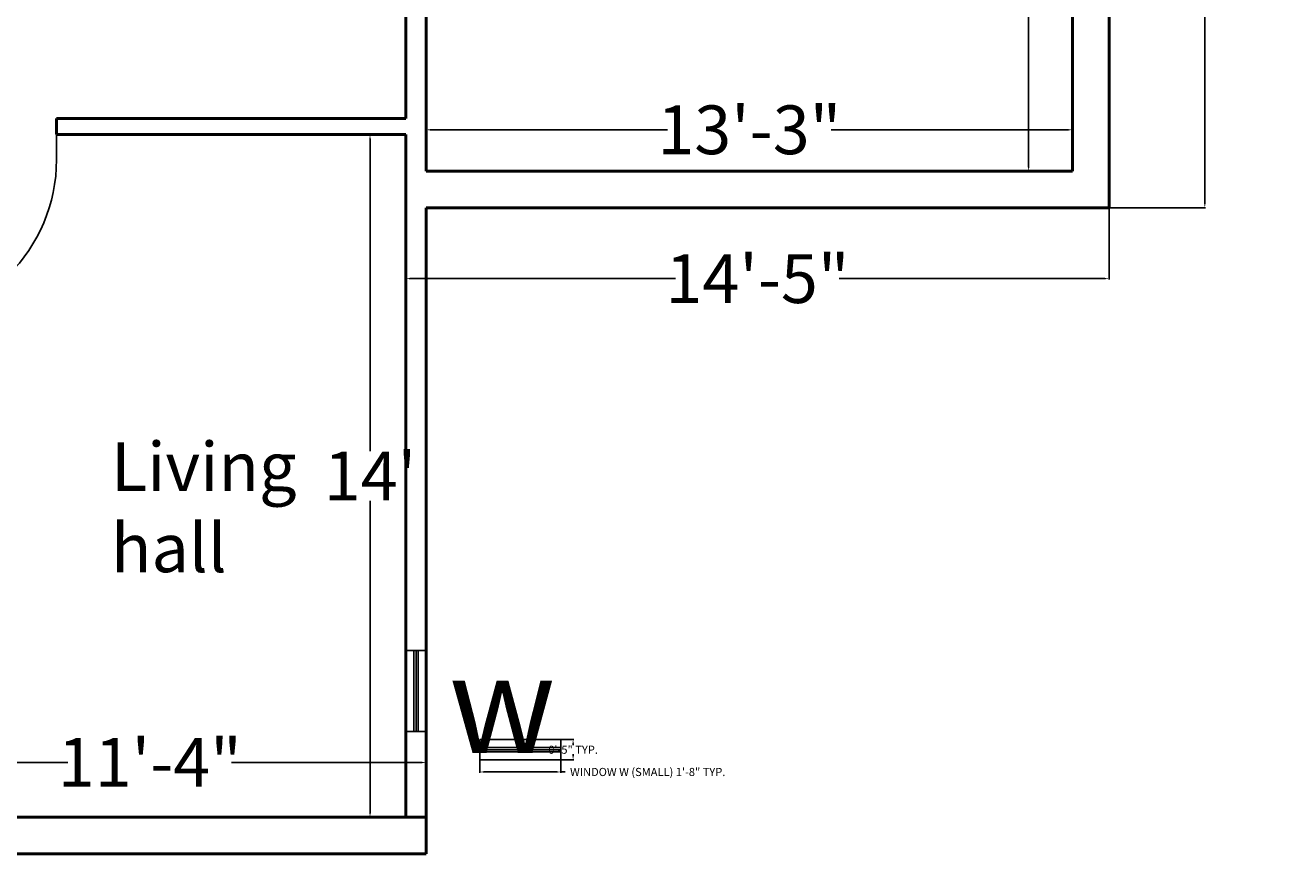
# Model space of a CAD drawing. Units: inches. Extents: x 409 to 7572, y 7 to 725.
# Tile 12 of 38: x 1972 to 2283, y 157 to 360. Entities that reach past the tile are written whole.
import ezdxf

# ---------------------------------------------------------------- set-up
doc = ezdxf.new("R2010")
doc.units = ezdxf.units.IN
doc.header["$MEASUREMENT"] = 0
for name, color, linetype, lineweight in [('A-ANNO-DIMS', 2, 'Continuous', 18), ('A-ANNO-SYMB', 3, 'Continuous', 25), ('A-AREA-IDEN', 7, 'Continuous', 25), ('A-DOOR', 3, 'Continuous', 25), ('A-GLAZ', 4, 'Continuous', 25), ('A-WALL', 7, 'Continuous', 50)]:
    doc.layers.add(name, color=color, linetype=linetype, lineweight=lineweight)
doc.styles.get("Standard").update_dxf_attribs({"font": 'arial.ttf'})
doc.dimstyles.get("Standard").update_dxf_attribs({"dimtxt": 2, "dimasz": 1, "dimexe": 0.18, "dimexo": 0.0625, "dimgap": 0.09, "dimtad": 0, "dimtih": 1, "dimtoh": 1, "dimdec": 0, "dimzin": 0, "dimdsep": 46, "dimlunit": 3, "dimtxsty": 'Standard', "dimcen": 0.09, "dimadec": 0, "dimazin": 0, "dimtfac": 1, "dimtdec": 0, "dimtofl": 0, "dimtmove": 0, "dimatfit": 3, "dimfxl": 1, "dimtolj": 1, "dimtzin": 0, "dimarcsym": 0})

# ---------------------------------------------------------------- blocks, each defined once
blk = doc.blocks.new('*U5')
for p, q in [((0, 0), (0, 6)), ((40, 0), (40, 6))]:
    blk.add_line(p, q)
blk.add_lwpolyline([(0, 0), (0, -40), (1.75, -40), (1.75, 0)], close=True)
blk.add_arc((0, 0), 40, 270, 0)
blk = doc.blocks.new('*D47')
at = {"layer": 'A-ANNO-DIMS', "color": 0, "lineweight": -2, "transparency": 16777216}
for p, q in [((2229.26, 444.53), (2218.37, 444.53)), ((2218.55, 443.53), (2218.55, 390.75)), ((2218.55, 325.53), (2218.55, 378.31)), ((2229.26, 324.53), (2218.37, 324.53))]:
    blk.add_line(p, q, dxfattribs=at)
at = {"layer": 'A-ANNO-DIMS', "color": 0, "transparency": 16777216}
for points in [[(2218.39, 443.53), (2218.72, 443.53), (2218.55, 444.53)], [(2218.39, 325.53), (2218.72, 325.53), (2218.55, 324.53)]]:
    blk.add_solid(points, dxfattribs=at)
at = {"layer": 'DEFPOINTS', "color": 0, "transparency": 16777216}
for p in [(2218.55, 444.53), (2229.32, 444.53), (2229.32, 324.53)]:
    blk.add_point(p, dxfattribs=at)
at = {"layer": 'A-ANNO-DIMS', "color": 0, "transparency": 16777216, "insert": (2218.55, 384.53), "char_height": 2, "attachment_point": 5}
blk.add_mtext("\\A1;{\\H6x;10'}", dxfattribs=at)
blk = doc.blocks.new('*D38')
at = {"layer": 'A-ANNO-DIMS', "color": 0, "lineweight": -2, "transparency": 16777216}
for p, q in [((2070.32, 324.59), (2070.32, 334.9)), ((2071.32, 334.72), (2129.68, 334.72)), ((2228.32, 334.72), (2169.96, 334.72)), ((2229.32, 324.59), (2229.32, 334.9))]:
    blk.add_line(p, q, dxfattribs=at)
at = {"layer": 'A-ANNO-DIMS', "color": 0, "transparency": 16777216}
for points in [[(2071.32, 334.88), (2071.32, 334.55), (2070.32, 334.72)], [(2228.32, 334.88), (2228.32, 334.55), (2229.32, 334.72)]]:
    blk.add_solid(points, dxfattribs=at)
at = {"layer": 'DEFPOINTS', "color": 0, "transparency": 16777216}
for p in [(2070.32, 334.72), (2070.32, 324.53), (2229.32, 324.53)]:
    blk.add_point(p, dxfattribs=at)
at = {"layer": 'A-ANNO-DIMS', "color": 0, "transparency": 16777216, "insert": (2149.82, 334.72), "char_height": 2, "attachment_point": 5}
blk.add_mtext('\\A1;{\\H6x;13\'-3"}', dxfattribs=at)
blk = doc.blocks.new('*D39')
at = {"layer": 'A-ANNO-DIMS', "color": 0, "lineweight": -2, "transparency": 16777216}
for p, q in [((2065.26, 333.53), (2056.33, 333.53)), ((2056.51, 332.53), (2056.51, 255.65)), ((2056.51, 166.53), (2056.51, 243.42)), ((2065.26, 165.53), (2056.33, 165.53))]:
    blk.add_line(p, q, dxfattribs=at)
at = {"layer": 'A-ANNO-DIMS', "color": 0, "transparency": 16777216}
for points in [[(2056.34, 332.53), (2056.67, 332.53), (2056.51, 333.53)], [(2056.34, 166.53), (2056.67, 166.53), (2056.51, 165.53)]]:
    blk.add_solid(points, dxfattribs=at)
at = {"layer": 'DEFPOINTS', "color": 0, "transparency": 16777216}
for p in [(2065.32, 333.53), (2056.51, 165.53), (2065.32, 165.53)]:
    blk.add_point(p, dxfattribs=at)
at = {"layer": 'A-ANNO-DIMS', "color": 0, "transparency": 16777216, "insert": (2056.51, 249.53), "char_height": 2, "attachment_point": 5}
blk.add_mtext("\\A1;{\\H6x;14'}", dxfattribs=at)
blk = doc.blocks.new('*D40')
at = {"layer": 'A-ANNO-DIMS', "color": 0, "lineweight": -2, "transparency": 16777216}
for p, q in [((1934.32, 165.59), (1934.32, 179.18)), ((1935.32, 179), (1982.18, 179)), ((2069.32, 179), (2022.46, 179)), ((2070.32, 165.59), (2070.32, 179.18))]:
    blk.add_line(p, q, dxfattribs=at)
at = {"layer": 'A-ANNO-DIMS', "color": 0, "transparency": 16777216}
for points in [[(1935.32, 179.16), (1935.32, 178.83), (1934.32, 179)], [(2069.32, 179.16), (2069.32, 178.83), (2070.32, 179)]]:
    blk.add_solid(points, dxfattribs=at)
at = {"layer": 'DEFPOINTS', "color": 0, "transparency": 16777216}
for p in [(2070.32, 179), (1934.32, 165.53), (2070.32, 165.53)]:
    blk.add_point(p, dxfattribs=at)
at = {"layer": 'A-ANNO-DIMS', "color": 0, "transparency": 16777216, "insert": (2002.32, 179), "char_height": 2, "attachment_point": 5}
blk.add_mtext('\\A1;{\\H6x;11\'-4"}', dxfattribs=at)
blk = doc.blocks.new('*D64')
at = {"layer": 'A-ANNO-DIMS', "color": 0, "lineweight": -2, "transparency": 16777216}
for p, q in [((2238.38, 672.53), (2262.07, 672.53)), ((2261.89, 671.53), (2261.89, 500.86)), ((2261.89, 316.53), (2261.89, 488.43)), ((2238.38, 315.53), (2262.07, 315.53))]:
    blk.add_line(p, q, dxfattribs=at)
at = {"layer": 'A-ANNO-DIMS', "color": 0, "transparency": 16777216}
for points in [[(2261.72, 671.53), (2262.05, 671.53), (2261.89, 672.53)], [(2261.72, 316.53), (2262.05, 316.53), (2261.89, 315.53)]]:
    blk.add_solid(points, dxfattribs=at)
at = {"layer": 'DEFPOINTS', "color": 0, "transparency": 16777216}
for p in [(2238.32, 672.53), (2261.89, 672.53), (2238.32, 315.53)]:
    blk.add_point(p, dxfattribs=at)
at = {"layer": 'A-ANNO-DIMS', "color": 0, "transparency": 16777216, "insert": (2261.89, 494.65), "char_height": 2, "attachment_point": 5}
blk.add_mtext('\\A1;{\\H6x;29\'-9"}', dxfattribs=at)
blk = doc.blocks.new('*D63')
at = {"layer": 'A-ANNO-DIMS', "color": 0, "lineweight": -2, "transparency": 16777216}
for p, q in [((2065.32, 315.37), (2065.32, 297.9)), ((2238.32, 315.37), (2238.32, 297.9)), ((2066.32, 298.08), (2131.68, 298.08)), ((2237.32, 298.08), (2171.96, 298.08))]:
    blk.add_line(p, q, dxfattribs=at)
at = {"layer": 'A-ANNO-DIMS', "color": 0, "transparency": 16777216}
for points in [[(2066.32, 298.25), (2066.32, 297.92), (2065.32, 298.08)], [(2237.32, 298.25), (2237.32, 297.92), (2238.32, 298.08)]]:
    blk.add_solid(points, dxfattribs=at)
at = {"layer": 'DEFPOINTS', "color": 0, "transparency": 16777216}
for p in [(2065.32, 315.43), (2238.32, 315.43), (2238.32, 298.08)]:
    blk.add_point(p, dxfattribs=at)
at = {"layer": 'A-ANNO-DIMS', "color": 0, "transparency": 16777216, "insert": (2151.82, 298.08), "char_height": 2, "attachment_point": 5}
blk.add_mtext('\\A1;{\\H6x;14\'-5"}', dxfattribs=at)
blk = doc.blocks.new('WIN-20')
for p, q in [((2103.48, 182.68), (2083.54, 182.68)), ((2103.48, 182.13), (2083.54, 182.13)), ((2103.48, 181.57), (2083.54, 181.57))]:
    blk.add_line(p, q)
blk.add_lwpolyline([(2103.48, 179.64), (2083.54, 179.64), (2083.54, 184.62), (2103.48, 184.62)], close=True)
blk = doc.blocks.new('*D171')
at = {"layer": 'A-ANNO-DIMS', "color": 0, "lineweight": -2, "transparency": 16777216}
for p, q in [((2083.54, 179.57), (2083.54, 176.47)), ((2103.48, 179.57), (2103.48, 176.47)), ((2084.54, 176.65), (2102.48, 176.65)), ((2103.48, 176.65), (2104.48, 176.65))]:
    blk.add_line(p, q, dxfattribs=at)
at = {"layer": 'A-ANNO-DIMS', "color": 0, "transparency": 16777216}
for points in [[(2084.54, 176.81), (2084.54, 176.48), (2083.54, 176.65)], [(2102.48, 176.81), (2102.48, 176.48), (2103.48, 176.65)]]:
    blk.add_solid(points, dxfattribs=at)
at = {"layer": 'DEFPOINTS', "color": 0, "transparency": 16777216}
for p in [(2083.54, 179.64), (2103.48, 179.64), (2103.48, 176.65)]:
    blk.add_point(p, dxfattribs=at)
at = {"layer": 'A-ANNO-DIMS', "color": 0, "transparency": 16777216, "insert": (2124.83, 176.65), "char_height": 2, "attachment_point": 5}
blk.add_mtext('\\A1;WINDOW W (SMALL) 1\'-8" TYP.', dxfattribs=at)
blk = doc.blocks.new('*D172')
at = {"layer": 'A-ANNO-DIMS', "color": 0, "lineweight": -2, "transparency": 16777216}
for p, q in [((2103.54, 184.62), (2106.65, 184.62)), ((2106.47, 183.62), (2106.47, 183.24)), ((2106.47, 180.64), (2106.47, 181.02)), ((2103.54, 179.64), (2106.65, 179.64))]:
    blk.add_line(p, q, dxfattribs=at)
at = {"layer": 'A-ANNO-DIMS', "color": 0, "transparency": 16777216}
for points in [[(2106.3, 183.62), (2106.63, 183.62), (2106.47, 184.62)], [(2106.3, 180.64), (2106.63, 180.64), (2106.47, 179.64)]]:
    blk.add_solid(points, dxfattribs=at)
at = {"layer": 'DEFPOINTS', "color": 0, "transparency": 16777216}
for p in [(2103.48, 184.62), (2106.47, 184.62), (2103.48, 179.64)]:
    blk.add_point(p, dxfattribs=at)
at = {"layer": 'A-ANNO-DIMS', "color": 0, "transparency": 16777216, "insert": (2106.47, 182.13), "char_height": 2, "attachment_point": 5}
blk.add_mtext('\\A1;0\'-5" TYP.', dxfattribs=at)

msp = doc.modelspace()

# ---------------------------------------------------------------- linework, layer by layer
at = {"layer": 'A-WALL'}
for p, q in [((2238.32, 315.53), (2238.32, 672.53)), ((2065.32, 525.53), (2065.32, 337.53)), ((2065.32, 489.53), (2065.32, 337.53)), ((2070.32, 444.53), (2070.32, 324.53)), ((2229.32, 324.53), (2229.32, 444.53)), ((1979.38, 337.53), (2065.32, 337.53)), ((1979.38, 337.53), (1979.38, 333.53)), ((1979.38, 333.53), (2065.32, 333.53)), ((2065.32, 333.53), (2065.32, 165.53)), ((2065.32, 333.53), (2065.32, 165.53)), ((2229.32, 324.53), (2070.32, 324.53)), ((2238.32, 315.53), (2070.32, 315.53)), ((2070.32, 315.53), (2070.32, 165.53)), ((1934.32, 165.53), (2070.32, 165.53)), ((2070.32, 165.53), (2070.32, 156.53)), ((1696.32, 156.53), (2070.32, 156.53))]:
    msp.add_line(p, q, dxfattribs=at)

# ---------------------------------------------------------------- block references
at = {"layer": 'A-DOOR'}
msp.add_blockref('*U5', (1939.38, 327.37), dxfattribs=at)
at = {"layer": 'A-GLAZ', "rotation": 89.99999999999905}
msp.add_blockref('WIN-20', (2249.96, -1896.94), dxfattribs=at)
at = {"layer": 'A-GLAZ'}
msp.add_blockref('WIN-20', (0, 0), dxfattribs=at)

# ---------------------------------------------------------------- texts
at = {"layer": 'A-ANNO-SYMB', "insert": (2075.9, 205.32), "char_height": 24, "attachment_point": 1}
msp.add_mtext_dynamic_manual_height_columns('w', width=18.2582, gutter_width=1, heights=[0], dxfattribs=at)
at = {"layer": 'A-AREA-IDEN', "insert": (1992.79, 257.83), "char_height": 12, "attachment_point": 1}
msp.add_mtext_dynamic_manual_height_columns('Living hall', width=58.8843, gutter_width=1, heights=[0], dxfattribs=at)

# ---------------------------------------------------------------- dimensions: what is measured, and where the dimension line sits
at = {"layer": 'A-ANNO-DIMS'}
dim = msp.add_linear_dim(base=(2261.89, 672.53), p1=(2238.32, 315.53), p2=(2238.32, 672.53), angle=90, text='{\\H6x;<>}', dimstyle='Standard', override={"dimclrd": 0, "dimclre": 0, "dimclrt": 0}, dxfattribs=at)
dim.commit()
dim.dimension.update_dxf_attribs({"geometry": '*D64', "text_midpoint": (2261.89, 494.65), "dimtype": 160})
for base, p1, p2, text, override, picture, middle in [((2218.55, 444.53), (2229.32, 324.53), (2229.32, 444.53), '{\\H6x;<>}', {"dimclrd": 0, "dimclre": 0, "dimclrt": 0}, '*D47', (2218.55, 384.53)), ((2056.51, 165.53), (2065.32, 333.53), (2065.32, 165.53), '{\\H6x;<>}', {"dimclrd": 0, "dimclre": 0, "dimclrt": 0}, '*D39', (2056.51, 249.53)), ((2106.47, 184.62), (2103.48, 179.64), (2103.48, 184.62), '<> TYP.', {"dimdec": 1, "dimrnd": 0, "dimzin": 1, "dimlunit": 4, "dimfrac": 2}, '*D172', (2106.47, 182.13))]:
    dim = msp.add_linear_dim(base=base, p1=p1, p2=p2, angle=90, text=text, dimstyle='Standard', override=override, dxfattribs=at)
    dim.commit()
    dim.dimension.update_dxf_attribs({"geometry": picture, "text_midpoint": middle})
for base, p1, p2, text, override, picture, middle in [((2070.32, 334.72), (2229.32, 324.53), (2070.32, 324.53), '{\\H6x;<>}', {"dimclrd": 0, "dimclre": 0, "dimclrt": 0}, '*D38', (2149.82, 334.72)), ((2238.32, 298.08), (2065.32, 315.43), (2238.32, 315.43), '{\\H6x;<>}', {"dimclrd": 0, "dimclre": 0, "dimclrt": 0}, '*D63', (2151.82, 298.08)), ((2070.32, 179), (1934.32, 165.53), (2070.32, 165.53), '{\\H6x;<>}', {"dimclrd": 0, "dimclre": 0, "dimclrt": 0}, '*D40', (2002.32, 179)), ((2103.48, 176.65), (2083.54, 179.64), (2103.48, 179.64), 'WINDOW W (SMALL) <> TYP.', {"dimdec": 1, "dimrnd": 0, "dimzin": 1, "dimlunit": 4, "dimfrac": 2}, '*D171', (2124.83, 176.65))]:
    dim = msp.add_linear_dim(base=base, p1=p1, p2=p2, text=text, dimstyle='Standard', override=override, dxfattribs=at)
    dim.commit()
    dim.dimension.update_dxf_attribs({"geometry": picture, "text_midpoint": middle})

doc.saveas('drawing.dxf')
